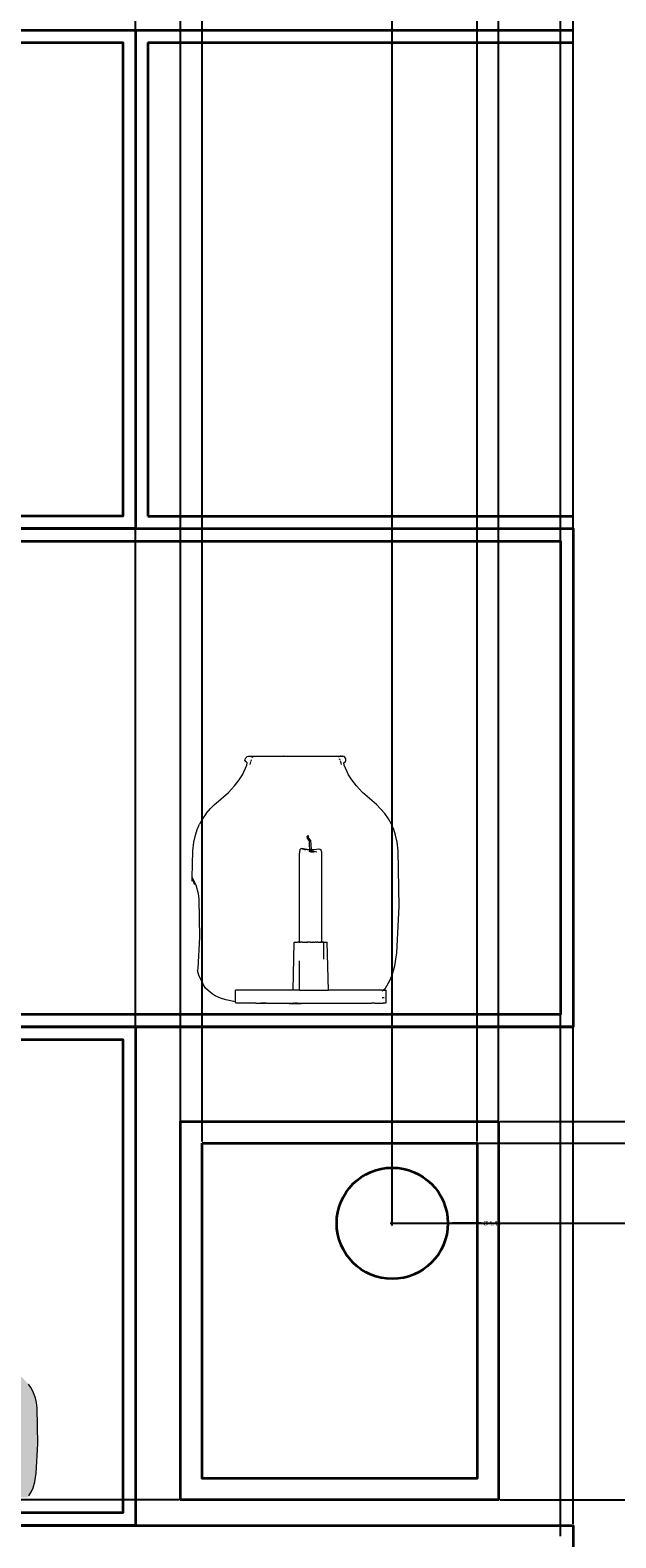
# Model space of a CAD drawing. Units: millimetres. Extents: x 446512 to 447461, y 70395 to 70610.
# Tile 19 of 39: x 446725 to 446748, y 70473 to 70533. Entities that reach past the tile are written whole.
import ezdxf

# ---------------------------------------------------------------- set-up
doc = ezdxf.new("R2010")
doc.units = ezdxf.units.MM
for name, color, linetype, lineweight in [('A-ANNO-DIMS', 2, 'Continuous', 18), ('A-FURN', 7, 'Continuous', 35), ('A-FURN-DECO', 8, 'Continuous', 13), ('A-FURN-PATT', 38, 'Continuous', 13)]:
    doc.layers.add(name, color=color, linetype=linetype, lineweight=lineweight)
doc.styles.get("Standard").update_dxf_attribs({"font": 'arial.ttf'})
doc.dimstyles.get("Standard").update_dxf_attribs({"dimtxt": 0.18, "dimasz": 0.18, "dimexe": 0.18, "dimexo": 0.0625, "dimgap": 0.09, "dimtad": 0, "dimtih": 1, "dimtoh": 1, "dimdec": 4, "dimzin": 0, "dimdsep": 46, "dimtxsty": 'Standard', "dimcen": 0.09, "dimadec": 0, "dimazin": 0, "dimtfac": 1, "dimtdec": 4, "dimtofl": 0, "dimtmove": 0, "dimatfit": 3, "dimfxl": 1, "dimtolj": 1, "dimtzin": 0, "dimarcsym": 0})

# ---------------------------------------------------------------- blocks, each defined once
blk = doc.blocks.new('DECO-VASE-B')
for p, q in [((2.121, 9.752), (2.128, 9.807)), ((2.121, 9.752), (2.136, 9.719)), ((2.128, 9.807), (2.158, 9.87)), ((2.184, 9.693), (2.136, 9.719)), ((2.158, 9.87), (2.204, 9.914)), ((2.208, 9.658), (2.184, 9.693)), ((2.204, 9.914), (2.257, 9.937)), ((2.257, 9.937), (2.375, 9.928)), ((2.257, 9.937), (3.651, 9.937)), ((2.34, 9.701), (2.323, 9.65)), ((2.369, 9.787), (2.35, 9.732)), ((2.375, 9.928), (2.419, 9.892)), ((2.419, 9.892), (2.422, 9.871)), ((3.666, 9.936), (3.651, 9.937)), ((3.666, 9.936), (5.973, 9.937)), ((5.872, 9.93), (5.946, 9.933)), ((5.899, 9.917), (5.879, 9.893)), ((5.891, 9.829), (5.92, 9.807)), ((5.946, 9.933), (5.899, 9.917)), ((5.92, 9.807), (5.927, 9.787)), ((5.944, 9.737), (5.948, 9.727)), ((5.973, 9.937), (5.946, 9.933)), ((5.954, 9.711), (5.974, 9.652)), ((5.977, 9.937), (5.973, 9.937)), ((5.977, 9.937), (6.043, 9.936)), ((6.097, 9.911), (6.043, 9.936)), ((6.151, 9.85), (6.097, 9.911)), ((6.097, 9.677), (6.158, 9.717)), ((6.169, 9.807), (6.151, 9.85)), ((6.158, 9.717), (6.174, 9.743)), ((6.174, 9.743), (6.169, 9.807)), ((1.892, 8.976), (2.026, 9.184)), ((2.026, 9.184), (2.196, 9.575)), ((2.196, 9.575), (2.208, 9.658)), ((2.323, 9.65), (2.313, 9.594)), ((5.974, 9.652), (5.984, 9.593)), ((6.088, 9.658), (6.097, 9.677)), ((6.101, 9.575), (6.088, 9.658)), ((6.27, 9.184), (6.101, 9.575)), ((6.405, 8.976), (6.27, 9.184)), ((0.966, 8.05), (1.454, 8.473)), ((1.454, 8.473), (1.704, 8.737)), ((1.704, 8.737), (1.892, 8.976)), ((6.592, 8.737), (6.405, 8.976)), ((6.842, 8.473), (6.592, 8.737)), ((7.4, 7.989), (6.842, 8.473)), ((0.741, 7.837), (0.896, 7.989)), ((0.896, 7.989), (0.966, 8.05)), ((7.734, 7.63), (7.4, 7.989)), ((0.415, 7.419), (0.296, 7.204)), ((0.562, 7.63), (0.415, 7.419)), ((0.562, 7.63), (0.741, 7.837)), ((7.882, 7.419), (7.734, 7.63)), ((8.001, 7.204), (7.882, 7.419)), ((0.066, 6.478), (0.13, 6.762)), ((0.13, 6.762), (0.202, 6.985)), ((0.202, 6.985), (0.296, 7.204)), ((4.665, 6.727), (4.616, 6.724)), ((4.628, 6.627), (4.616, 6.724)), ((4.676, 6.66), (4.665, 6.727)), ((4.753, 6.557), (4.676, 6.66)), ((8.095, 6.985), (8.001, 7.204)), ((8.167, 6.762), (8.095, 6.985)), ((8.23, 6.478), (8.167, 6.762)), ((0.003, 5.065), (0.022, 6.129)), ((0.022, 6.129), (0.066, 6.478)), ((4.307, 5.974), (4.332, 6.194)), ((4.392, 6.222), (4.332, 6.194)), ((4.611, 6.182), (4.392, 6.222)), ((4.567, 6.159), (4.412, 6.207)), ((4.412, 6.207), (4.611, 6.182)), ((4.611, 6.182), (4.719, 6.182)), ((4.72, 6.153), (4.611, 6.182)), ((4.711, 6.536), (4.628, 6.627)), ((4.721, 6.111), (4.691, 6.12)), ((4.714, 6.371), (4.711, 6.536)), ((4.719, 6.182), (4.714, 6.371)), ((4.72, 6.153), (4.719, 6.182)), ((4.719, 6.182), (4.779, 6.182)), ((4.782, 6.137), (4.72, 6.153)), ((4.72, 6.143), (4.72, 6.149)), ((4.721, 6.111), (4.721, 6.13)), ((4.752, 6.101), (4.721, 6.111)), ((4.722, 6.089), (4.721, 6.111)), ((4.761, 6.087), (4.722, 6.089)), ((4.752, 6.101), (4.784, 6.098)), ((4.753, 6.557), (4.779, 6.182)), ((4.761, 6.087), (4.785, 6.086)), ((4.779, 6.182), (4.782, 6.137)), ((4.779, 6.182), (4.892, 6.182)), ((5.006, 6.08), (4.782, 6.137)), ((4.782, 6.129), (4.783, 6.109)), ((4.784, 6.098), (4.785, 6.086)), ((4.784, 6.098), (4.899, 6.089)), ((4.892, 6.182), (5.091, 6.212)), ((5.091, 6.212), (5.171, 6.181)), ((5.19, 6.109), (5.171, 6.181)), ((5.19, 6.109), (5.194, 2.461)), ((8.274, 6.129), (8.23, 6.478)), ((8.315, 3.894), (8.274, 6.129)), ((4.307, 2.461), (4.307, 5.974)), ((0, 4.992), (0.003, 5.065)), ((0.002, 4.989), (0, 4.992)), ((0, 4.911), (0.002, 4.989)), ((0.057, 4.898), (0.002, 4.989)), ((0.003, 5.065), (0.148, 4.769)), ((0.105, 4.769), (0.057, 4.898)), ((0.148, 4.769), (0.24, 4.424)), ((0.24, 4.424), (0.27, 4.187)), ((0.27, 4.187), (0.298, 2.664)), ((8.221, 2.044), (8.315, 3.894)), ((0.298, 2.664), (0.234, 1.404)), ((4.054, 0.538), (4.098, 2.454)), ((4.098, 2.454), (4.106, 2.461)), ((4.106, 2.461), (4.163, 2.461)), ((4.163, 2.461), (4.167, 2.461)), ((4.167, 2.461), (4.192, 2.461)), ((4.192, 2.461), (4.198, 2.461)), ((4.198, 2.461), (4.201, 2.461)), ((4.201, 2.461), (4.218, 2.461)), ((4.218, 2.461), (4.227, 2.461)), ((4.227, 2.461), (4.232, 2.461)), ((4.232, 2.461), (4.235, 2.461)), ((4.235, 2.461), (4.239, 2.461)), ((4.239, 2.461), (4.246, 2.461)), ((4.25, 2.461), (4.246, 2.461)), ((4.246, 2.461), (4.246, 2.454)), ((4.25, 2.461), (4.253, 2.461)), ((4.253, 2.461), (4.261, 2.461)), ((4.274, 2.461), (4.261, 2.461)), ((4.278, 2.461), (4.274, 2.461)), ((4.278, 2.461), (4.29, 2.461)), ((4.29, 2.461), (4.293, 2.461)), ((4.293, 2.461), (4.295, 2.461)), ((4.295, 2.461), (4.307, 2.461)), ((4.307, 2.454), (4.307, 2.461)), ((4.323, 2.461), (4.307, 2.461)), ((4.323, 2.461), (4.344, 2.461)), ((4.416, 2.461), (4.344, 2.461)), ((4.427, 2.461), (4.416, 2.461)), ((4.427, 2.461), (4.484, 2.461)), ((4.484, 2.461), (4.498, 2.461)), ((4.498, 2.461), (4.589, 2.461)), ((4.605, 2.461), (4.589, 2.461)), ((4.605, 2.461), (4.638, 2.461)), ((4.732, 2.461), (4.638, 2.461)), ((4.732, 2.461), (4.738, 2.461)), ((4.738, 2.461), (4.839, 2.461)), ((4.861, 2.461), (4.839, 2.461)), ((4.861, 2.461), (4.924, 2.461)), ((4.924, 2.461), (4.937, 2.461)), ((4.973, 2.461), (4.937, 2.461)), ((4.978, 2.461), (4.973, 2.461)), ((4.983, 2.461), (4.978, 2.461)), ((4.983, 2.461), (4.987, 2.461)), ((4.987, 2.461), (4.99, 2.461)), ((4.99, 2.461), (5.024, 2.461)), ((5.037, 2.461), (5.024, 2.461)), ((5.064, 2.461), (5.037, 2.461)), ((5.064, 2.461), (5.07, 2.461)), ((5.07, 2.461), (5.144, 2.461)), ((5.154, 2.461), (5.144, 2.461)), ((5.154, 2.461), (5.181, 2.461)), ((5.188, 2.461), (5.181, 2.461)), ((5.194, 2.461), (5.188, 2.461)), ((5.194, 2.461), (5.194, 2.454)), ((5.196, 2.461), (5.194, 2.461)), ((5.202, 2.461), (5.196, 2.461)), ((5.204, 2.461), (5.202, 2.461)), ((5.204, 2.461), (5.219, 2.461)), ((5.224, 2.461), (5.219, 2.461)), ((5.244, 2.461), (5.224, 2.461)), ((5.249, 2.461), (5.244, 2.461)), ((5.249, 2.461), (5.262, 2.461)), ((5.276, 2.461), (5.262, 2.461)), ((5.276, 2.461), (5.266, 1.782)), ((5.28, 2.461), (5.276, 2.461)), ((5.285, 2.461), (5.28, 2.461)), ((5.285, 2.461), (5.312, 2.461)), ((5.312, 2.461), (5.318, 2.461)), ((5.318, 2.461), (5.325, 2.461)), ((5.325, 2.461), (5.348, 2.461)), ((5.348, 2.461), (5.351, 2.461)), ((5.351, 2.461), (5.355, 2.461)), ((5.355, 2.461), (5.365, 2.461)), ((5.365, 2.461), (5.415, 2.461)), ((5.423, 2.454), (5.415, 2.461)), ((5.467, 0.538), (5.423, 2.454)), ((8.128, 1.516), (8.221, 2.044)), ((0.234, 1.404), (0.221, 1.331)), ((0.275, 1.141), (0.221, 1.331)), ((4.307, 0.538), (4.307, 1.712)), ((8.022, 1.141), (8.128, 1.516)), ((0.453, 0.752), (0.275, 1.141)), ((0.54, 0.627), (0.453, 0.752)), ((0.637, 0.522), (0.54, 0.627)), ((7.662, 0.538), (7.756, 0.627)), ((7.756, 0.627), (7.921, 0.896)), ((7.921, 0.896), (8.022, 1.141)), ((0.804, 0.392), (0.637, 0.522)), ((0.929, 0.318), (0.804, 0.392)), ((1.134, 0.226), (0.929, 0.318)), ((1.358, 0.154), (1.134, 0.226)), ((1.679, 0.085), (1.358, 0.154)), ((1.734, 0.078), (1.679, 0.085)), ((1.734, 0.266), (1.734, 0.538)), ((4.054, 0.538), (1.734, 0.538)), ((1.734, 0.078), (1.734, 0.266)), ((1.734, 0.049), (1.734, 0.078)), ((1.757, 0.021), (1.734, 0.049)), ((2.515, 0.021), (1.757, 0.021)), ((2.539, 0.023), (2.515, 0.021)), ((2.551, 0.021), (2.539, 0.023)), ((2.551, 0.021), (2.948, 0.021)), ((2.948, 0.021), (2.761, 0.023)), ((2.969, 0.024), (2.948, 0.021)), ((2.991, 0.021), (2.969, 0.024)), ((2.991, 0.021), (4.067, 0.021)), ((3.896, 0), (4.077, 0.018)), ((4.307, 0.538), (4.054, 0.538)), ((4.077, 0.018), (4.067, 0.021)), ((4.077, 0.018), (4.126, 0.021)), ((4.176, 0.018), (4.126, 0.021)), ((4.196, 0.021), (4.176, 0.018)), ((4.196, 0.021), (4.248, 0.018)), ((4.248, 0.018), (4.27, 0.021)), ((4.392, 0), (4.248, 0.018)), ((4.27, 0.021), (7.006, 0.021)), ((4.307, 0.538), (5.467, 0.538)), ((7.621, 0.538), (5.467, 0.538)), ((7.006, 0.021), (7.192, 0.022)), ((7.325, 0.021), (7.192, 0.022)), ((7.325, 0.021), (7.349, 0.022)), ((7.349, 0.022), (7.351, 0.022)), ((7.349, 0.022), (7.353, 0.022)), ((7.353, 0.022), (7.467, 0.021)), ((7.467, 0.021), (7.488, 0.022)), ((7.488, 0.022), (7.49, 0.022)), ((7.49, 0.022), (7.582, 0.021)), ((7.582, 0.021), (7.645, 0.021)), ((7.621, 0.499), (7.662, 0.538)), ((7.621, 0.538), (7.662, 0.538)), ((7.645, 0.021), (7.67, 0.021)), ((7.675, 0.538), (7.662, 0.538)), ((7.683, 0.021), (7.67, 0.021)), ((7.692, 0.538), (7.675, 0.538)), ((7.765, 0.021), (7.683, 0.021)), ((7.692, 0.538), (7.787, 0.538)), ((7.765, 0.021), (7.788, 0.049)), ((7.788, 0.049), (7.787, 0.538)), ((3.896, 0), (4.392, 0))]:
    blk.add_line(p, q)
blk = doc.blocks.new('*D29')
at = {"layer": 'A-ANNO-DIMS', "color": 0, "lineweight": -2, "transparency": 16777216}
for p, q in [((446730.822, 70489.647), (446730.822, 70578.175)), ((446743.582, 70489.647), (446743.582, 70578.175)), ((446731.002, 70577.995), (446736.817, 70577.995)), ((446743.402, 70577.995), (446737.587, 70577.995))]:
    blk.add_line(p, q, dxfattribs=at)
at = {"layer": 'A-ANNO-DIMS', "color": 0, "transparency": 16777216}
for points in [[(446731.002, 70578.025), (446731.002, 70577.965), (446730.822, 70577.995)], [(446743.402, 70578.025), (446743.402, 70577.965), (446743.582, 70577.995)]]:
    blk.add_solid(points, dxfattribs=at)
at = {"layer": 'Defpoints', "color": 0, "transparency": 16777216}
for p in [(446743.582, 70577.995), (446730.822, 70489.584), (446743.582, 70489.584)]:
    blk.add_point(p, dxfattribs=at)
at = {"layer": 'A-ANNO-DIMS', "color": 0, "transparency": 16777216, "insert": (446737.202, 70577.995), "char_height": 0.18, "attachment_point": 5}
blk.add_mtext('\\A1;12.76', dxfattribs=at)
blk = doc.blocks.new('*D30')
at = {"layer": 'A-ANNO-DIMS', "color": 0, "lineweight": -2, "transparency": 16777216}
for p, q in [((446743.644, 70489.584), (446787.753, 70489.584)), ((446787.573, 70489.404), (446787.573, 70482.176)), ((446787.573, 70474.585), (446787.573, 70481.813)), ((446743.644, 70474.405), (446787.753, 70474.405))]:
    blk.add_line(p, q, dxfattribs=at)
at = {"layer": 'A-ANNO-DIMS', "color": 0, "transparency": 16777216}
for points in [[(446787.543, 70489.404), (446787.603, 70489.404), (446787.573, 70489.584)], [(446787.543, 70474.585), (446787.603, 70474.585), (446787.573, 70474.405)]]:
    blk.add_solid(points, dxfattribs=at)
at = {"layer": 'Defpoints', "color": 0, "transparency": 16777216}
for p in [(446743.582, 70489.584), (446787.573, 70489.584), (446743.582, 70474.405)]:
    blk.add_point(p, dxfattribs=at)
at = {"layer": 'A-ANNO-DIMS', "color": 0, "transparency": 16777216, "insert": (446787.573, 70481.995), "char_height": 0.18, "attachment_point": 5}
blk.add_mtext('\\A1;15.18', dxfattribs=at)
blk = doc.blocks.new('*D31')
at = {"layer": 'A-ANNO-DIMS', "color": 0, "lineweight": -2, "transparency": 16777216}
for p, q in [((446729.008, 70473.444), (446729.008, 70578.175)), ((446730.822, 70474.467), (446730.822, 70578.175)), ((446729.188, 70577.995), (446729.531, 70577.995)), ((446730.642, 70577.995), (446730.3, 70577.995))]:
    blk.add_line(p, q, dxfattribs=at)
at = {"layer": 'A-ANNO-DIMS', "color": 0, "transparency": 16777216}
for points in [[(446729.188, 70578.025), (446729.188, 70577.965), (446729.008, 70577.995)], [(446730.642, 70578.025), (446730.642, 70577.965), (446730.822, 70577.995)]]:
    blk.add_solid(points, dxfattribs=at)
at = {"layer": 'Defpoints', "color": 0, "transparency": 16777216}
for p in [(446730.822, 70577.995), (446730.822, 70474.405), (446729.008, 70473.382)]:
    blk.add_point(p, dxfattribs=at)
at = {"layer": 'A-ANNO-DIMS', "color": 0, "transparency": 16777216, "insert": (446729.915, 70577.995), "char_height": 0.18, "attachment_point": 5}
blk.add_mtext('\\A1;1.814', dxfattribs=at)
blk = doc.blocks.new('*D32')
at = {"layer": 'A-ANNO-DIMS', "color": 0, "lineweight": -2, "transparency": 16777216}
for p, q in [((446730.76, 70474.405), (446678.043, 70474.405)), ((446678.223, 70474.225), (446678.223, 70474.075)), ((446678.223, 70473.562), (446678.223, 70473.711)), ((446728.946, 70473.382), (446678.043, 70473.382))]:
    blk.add_line(p, q, dxfattribs=at)
at = {"layer": 'A-ANNO-DIMS', "color": 0, "transparency": 16777216}
for points in [[(446678.193, 70474.225), (446678.253, 70474.225), (446678.223, 70474.405)], [(446678.193, 70473.562), (446678.253, 70473.562), (446678.223, 70473.382)]]:
    blk.add_solid(points, dxfattribs=at)
at = {"layer": 'Defpoints', "color": 0, "transparency": 16777216}
for p in [(446730.822, 70474.405), (446678.223, 70473.382), (446729.008, 70473.382)]:
    blk.add_point(p, dxfattribs=at)
at = {"layer": 'A-ANNO-DIMS', "color": 0, "transparency": 16777216, "insert": (446678.223, 70473.893), "char_height": 0.18, "attachment_point": 5}
blk.add_mtext('\\A1;1.02', dxfattribs=at)
blk = doc.blocks.new('*D33')
at = {"layer": 'A-ANNO-DIMS', "color": 0, "lineweight": -2, "transparency": 16777216}
for p, q in [((446730.822366, 70489.64696), (446730.822366, 70578.17492)), ((446731.68472, 70488.784606), (446731.68472, 70578.17492)), ((446730.642366, 70577.99492), (446730.462366, 70577.99492)), ((446731.86472, 70577.99492), (446732.04472, 70577.99492))]:
    blk.add_line(p, q, dxfattribs=at)
at = {"layer": 'A-ANNO-DIMS', "color": 0, "transparency": 16777216}
for points in [[(446730.642366, 70578.02492), (446730.642366, 70577.96492), (446730.822366, 70577.99492)], [(446731.86472, 70578.02492), (446731.86472, 70577.96492), (446731.68472, 70577.99492)]]:
    blk.add_solid(points, dxfattribs=at)
at = {"layer": 'Defpoints', "color": 0, "transparency": 16777216}
for p in [(446731.68472, 70577.99492), (446730.822366, 70489.58446), (446731.68472, 70488.722106)]:
    blk.add_point(p, dxfattribs=at)
at = {"layer": 'A-ANNO-DIMS', "color": 0, "transparency": 16777216, "insert": (446731.253543, 70577.99492), "char_height": 0.18, "attachment_point": 5}
blk.add_mtext('\\A1;0.86', dxfattribs=at)
blk = doc.blocks.new('*D34')
at = {"layer": 'A-ANNO-DIMS', "color": 0, "lineweight": -2, "transparency": 16777216}
for p, q in [((446739.318, 70485.567), (446739.318, 70578.175)), ((446742.719, 70488.785), (446742.719, 70578.175)), ((446739.498, 70577.995), (446740.642, 70577.995)), ((446742.539, 70577.995), (446741.395, 70577.995))]:
    blk.add_line(p, q, dxfattribs=at)
at = {"layer": 'A-ANNO-DIMS', "color": 0, "transparency": 16777216}
for points in [[(446739.498, 70578.025), (446739.498, 70577.965), (446739.318, 70577.995)], [(446742.539, 70578.025), (446742.539, 70577.965), (446742.719, 70577.995)]]:
    blk.add_solid(points, dxfattribs=at)
at = {"layer": 'Defpoints', "color": 0, "transparency": 16777216}
for p in [(446739.318, 70577.995), (446742.719, 70488.722), (446739.318, 70485.504)]:
    blk.add_point(p, dxfattribs=at)
at = {"layer": 'A-ANNO-DIMS', "color": 0, "transparency": 16777216, "insert": (446741.019, 70577.995), "char_height": 0.18, "attachment_point": 5}
blk.add_mtext('\\A1;3.401', dxfattribs=at)
blk = doc.blocks.new('*D35')
at = {"layer": 'A-ANNO-DIMS', "color": 0, "lineweight": -2, "transparency": 16777216}
for p, q in [((446742.782, 70488.722), (446787.753, 70488.722)), ((446787.573, 70488.542), (446787.573, 70487.295)), ((446787.573, 70485.684), (446787.573, 70486.931)), ((446739.381, 70485.504), (446787.753, 70485.504))]:
    blk.add_line(p, q, dxfattribs=at)
at = {"layer": 'A-ANNO-DIMS', "color": 0, "transparency": 16777216}
for points in [[(446787.543, 70488.542), (446787.603, 70488.542), (446787.573, 70488.722)], [(446787.543, 70485.684), (446787.603, 70485.684), (446787.573, 70485.504)]]:
    blk.add_solid(points, dxfattribs=at)
at = {"layer": 'Defpoints', "color": 0, "transparency": 16777216}
for p in [(446742.719, 70488.722), (446739.318, 70485.504), (446787.573, 70485.504)]:
    blk.add_point(p, dxfattribs=at)
at = {"layer": 'A-ANNO-DIMS', "color": 0, "transparency": 16777216, "insert": (446787.573, 70487.113), "char_height": 0.18, "attachment_point": 5}
blk.add_mtext('\\A1;3.22', dxfattribs=at)
blk = doc.blocks.new('*D36')
at = {"layer": 'A-ANNO-DIMS', "color": 0, "lineweight": -2, "transparency": 16777216}
for p, q in [((446746.073, 70472.944), (446746.073, 70578.175)), ((446746.573, 70473.444), (446746.573, 70578.175)), ((446745.893, 70577.995), (446745.713, 70577.995)), ((446746.753, 70577.995), (446746.933, 70577.995))]:
    blk.add_line(p, q, dxfattribs=at)
at = {"layer": 'A-ANNO-DIMS', "color": 0, "transparency": 16777216}
for points in [[(446745.893, 70578.025), (446745.893, 70577.965), (446746.073, 70577.995)], [(446746.753, 70578.025), (446746.753, 70577.965), (446746.573, 70577.995)]]:
    blk.add_solid(points, dxfattribs=at)
at = {"layer": 'Defpoints', "color": 0, "transparency": 16777216}
for p in [(446746.573, 70577.995), (446746.073, 70472.882), (446746.573, 70473.382)]:
    blk.add_point(p, dxfattribs=at)
at = {"layer": 'A-ANNO-DIMS', "color": 0, "transparency": 16777216, "insert": (446747.187, 70577.995), "char_height": 0.18, "attachment_point": 5}
blk.add_mtext('\\A1;0.5', dxfattribs=at)
blk = doc.blocks.new('*D78')
at = {"layer": 'A-ANNO-DIMS', "color": 0, "lineweight": -2, "transparency": 16777216}
for p, q in [((446739.318, 70485.414), (446739.318, 70485.594)), ((446739.228, 70485.504), (446739.408, 70485.504)), ((446742.886, 70485.504), (446741.728, 70485.504))]:
    blk.add_line(p, q, dxfattribs=at)
at = {"layer": 'A-ANNO-DIMS', "color": 0, "transparency": 16777216}
blk.add_solid([(446741.728, 70485.534), (446741.728, 70485.474), (446741.548, 70485.504)], dxfattribs=at)
at = {"layer": 'Defpoints', "color": 0, "transparency": 16777216}
for p in [(446737.088, 70485.505), (446741.548, 70485.504)]:
    blk.add_point(p, dxfattribs=at)
at = {"layer": 'A-ANNO-DIMS', "color": 0, "transparency": 16777216, "insert": (446743.308, 70485.504), "char_height": 0.18, "attachment_point": 5}
blk.add_mtext('\\A1;∅4.46', dxfattribs=at)

msp = doc.modelspace()

# ---------------------------------------------------------------- hatches: boundary and pattern name
at = {"layer": 'A-FURN-PATT'}
h = msp.add_hatch(color=256, dxfattribs=at)
h.dxf.hatch_style = 1
h.paths.add_polyline_path([(446703.5722, 70477.5476), (446703.5295, 70477.5904), (446703.508, 70477.5904), (446703.383, 70477.6041), (446703.3062, 70477.6039), (446702.8621, 70477.6193), (446702.7177, 70477.6193), (446702.6174, 70477.6163), (446702.576, 70477.615), (446702.5757, 70477.6192), (446702.3373, 70477.6192), (446701.7238, 70477.5898), (446701.6039, 70477.5792), (446701.5612, 70477.5357), (446701.547, 70474.1653), (446703.5225, 70474.1653), (446703.5865, 70474.1653), (446703.5861, 70474.2632), (446703.5852, 70474.4594)])
h.paths.add_polyline_path([(446715.9764, 70475.5286), (446716.1565, 70476.0766), (446716.2492, 70476.4728), (446716.2873, 70476.8422), (446716.2666, 70477.0104), (446716.236, 70477.1061), (446716.1173, 70477.332), (446715.9979, 70477.4937), (446715.8249, 70477.6853), (446715.558, 70477.9316), (446715.2321, 70478.1882), (446714.7182, 70478.5467), (446714.5954, 70478.6535), (446714.3996, 70478.8999), (446714.3461, 70479.0185), (446714.3253, 70479.1028), (446714.3286, 70480.1095), (446714.368, 70480.1364), (446714.3744, 70480.152), (446714.3709, 70480.1808), (446714.3551, 70480.2131), (446714.3271, 70480.2359), (446714.3039, 70480.2478), (446714.2782, 70480.2478), (446714.259, 70480.2458), (446714.2432, 70480.2391), (446714.2375, 70480.2284), (446714.2369, 70480.2218), (446714.2301, 70480.2478), (446713.8255, 70480.2478), (446713.8277, 70480.2375), (446713.8104, 70480.2458), (446713.7912, 70480.2478), (446713.7655, 70480.2478), (446713.738, 70480.2359), (446713.7079, 70480.2028), (446713.6947, 70480.1567), (446713.6986, 70480.1448), (446713.717, 70480.1274), (446713.7341, 70480.1112), (446713.7407, 70480.1049), (446713.7473, 70479.1348), (446713.7233, 70479.0185), (446713.6698, 70478.8999), (446713.5684, 70478.7546), (446713.4739, 70478.6535), (446713.3511, 70478.5467), (446712.8373, 70478.1882), (446712.5114, 70477.9316), (446712.4629, 70477.8868), (446712.2445, 70477.6853), (446712.0714, 70477.4937), (446711.9521, 70477.332), (446711.866, 70477.1682), (446711.8333, 70477.1061), (446711.7899, 70476.9473), (446711.7821, 70476.8422), (446711.8202, 70476.4728), (446711.8563, 70476.3184), (446711.9128, 70476.0766), (446712.093, 70475.5286), (446712.2916, 70475.0627), (446712.4529, 70474.7607), (446712.5622, 70474.5947), (446712.6434, 70474.4935), (446712.7522, 70474.3925), (446712.8451, 70474.3334), (446713.0597, 70474.2483), (446713.2189, 70474.2124), (446713.4296, 70474.1861), (446713.8128, 70474.1834), (446713.5915, 70474.1683), (446714.5392, 70474.1683), (446714.4414, 70474.1779), (446714.1836, 70474.1834), (446714.6098, 70474.1861), (446714.8353, 70474.2124), (446714.9266, 70474.2312), (446715.0097, 70474.2483), (446715.2243, 70474.3334), (446715.3172, 70474.3925), (446715.3727, 70474.4388), (446715.5072, 70474.5947), (446715.6164, 70474.7607), (446715.7778, 70475.0627)])
h.paths.add_polyline_path([(446719.9646, 70475.8685), (446719.9469, 70476.8426), (446719.9277, 70476.9944), (446719.8688, 70477.2155), (446719.7757, 70477.4048), (446719.7115, 70477.4967), (446719.566, 70477.6531), (446719.2165, 70477.9493), (446719.1289, 70478.0481), (446719.1777, 70478.067), (446719.1866, 70478.0815), (446719.1867, 70478.209), (446719.1598, 70478.218), (446719.1369, 70478.2173), (446719.1374, 70478.2174), (446719.0341, 70478.2174), (446718.8666, 70478.218), (446718.6447, 70478.218), (446718.418, 70478.2174), (446718.1448, 70478.2174), (446717.8911, 70478.218), (446717.8873, 70478.218), (446717.6401, 70478.2174), (446717.4215, 70478.2174), (446717.2754, 70478.218), (446717.1987, 70478.218), (446717.2097, 70478.2113), (446717.1243, 70478.2174), (446717.1135, 70478.2124), (446717.1091, 70478.2029), (446717.1111, 70478.0815), (446717.1185, 70478.0683), (446717.1615, 70478.0517), (446717.1433, 70478.0167), (446717.0812, 70477.9493), (446716.7317, 70477.6531), (446716.5862, 70477.4967), (446716.47, 70477.311), (446716.3975, 70477.1183), (446716.37, 70476.9944), (446716.3508, 70476.8426), (446716.3331, 70475.8685), (446716.374, 70475.0624), (446716.4146, 70474.8322), (446716.4608, 70474.6687), (446716.5046, 70474.5619), (446716.5765, 70474.4449), (446716.6659, 70474.36), (446716.7457, 70474.3103), (446716.8351, 70474.2702), (446717.0729, 70474.2085), (446717.2886, 70474.1864), (446717.3803, 70474.1864), (446717.4428, 70474.1846), (446717.4556, 70474.1862), (446718.0146, 70474.1842), (446718.1072, 70474.1795), (446718.1371, 70474.1802), (446718.1473, 70474.1804), (446718.1566, 70474.1797), (446718.1569, 70474.1797), (446718.1592, 70474.1795), (446718.303, 70474.1842), (446719.0393, 70474.1865), (446719.2248, 70474.2085), (446719.365, 70474.2387), (446719.4626, 70474.2702), (446719.552, 70474.3103), (446719.6318, 70474.36), (446719.7212, 70474.4449), (446719.7931, 70474.5619), (446719.8369, 70474.6687), (446719.8831, 70474.8322), (446719.9155, 70475.0156), (446719.9237, 70475.0624)])
h.paths.add_polyline_path([(446718.18, 70474.3158), (446717.2692, 70474.3158), (446717.2092, 70474.3107), (446717.3763, 70474.3107)], flags=16)
h.paths.add_polyline_path([(446717.572, 70474.3384), (446717.5676, 70474.3381), (446717.5691, 70474.3381)], flags=16)
h.paths.add_polyline_path([(446722.3965, 70475.7383), (446722.4453, 70475.7383), (446722.4564, 70475.7383), (446722.4729, 70475.7383), (446722.4785, 70475.7384), (446722.4797, 70475.7383), (446722.4831, 70475.7383), (446722.4841, 70475.7384), (446722.5211, 70475.7384), (446722.4906, 70475.7381), (446722.4906, 70475.7384), (446722.4864, 70475.7383), (446722.4853, 70475.7383), (446722.4831, 70475.7383), (446722.4819, 70475.7383), (446722.4797, 70475.7383), (446722.4618, 70475.7383), (446722.4401, 70475.7383), (446722.4015, 70475.7383), (446722.3964, 70475.7341), (446722.3682, 70474.5084), (446722.5299, 70474.5084), (446723.2721, 70474.5084), (446723.2439, 70475.7341), (446723.2391, 70475.7383), (446723.2067, 70475.7383), (446723.1904, 70475.7383), (446723.1824, 70475.7383), (446723.1499, 70475.7382), (446723.1499, 70475.7384), (446723.1407, 70475.7384), (446723.1819, 70475.7384), (446723.1732, 70475.7384), (446723.1824, 70475.7383), (446723.1957, 70475.7383), (446723.1982, 70475.7383), (446723.2002, 70475.7383), (446723.2067, 70475.7383), (446723.2439, 70475.7383), (446723.2721, 70474.5084), (446724.6768, 70474.5084), (446724.7369, 70474.5652), (446724.8426, 70474.7369), (446724.9068, 70474.8938), (446724.9747, 70475.1338), (446725.0344, 70475.4718), (446725.0943, 70476.6554), (446725.0683, 70478.0856), (446725.0402, 70478.3085), (446724.9998, 70478.4903), (446724.9537, 70478.6331), (446724.8934, 70478.7733), (446724.817, 70478.911), (446724.7228, 70479.046), (446724.5091, 70479.2756), (446724.1522, 70479.5853), (446723.9922, 70479.7544), (446723.8721, 70479.9071), (446723.7862, 70480.0401), (446723.6778, 70480.2901), (446723.6684, 70480.351), (446723.714, 70480.381), (446723.7245, 70480.398), (446723.7213, 70480.4391), (446723.7096, 70480.4663), (446723.6751, 70480.5056), (446723.6405, 70480.5215), (446723.5985, 70480.5218), (446723.5958, 70480.5218), (446722.1196, 70480.5215), (446721.2867, 70480.5218), (446721.2939, 70480.516), (446721.2184, 70480.5218), (446721.1844, 70480.5072), (446721.155, 70480.479), (446721.1354, 70480.4391), (446721.1312, 70480.4035), (446721.1408, 70480.3826), (446721.1891, 70480.3558), (446721.179, 70480.2901), (446721.0706, 70480.0401), (446720.9847, 70479.9071), (446720.8645, 70479.7544), (446720.7046, 70479.5853), (446720.3925, 70479.3145), (446720.3476, 70479.2756), (446720.248, 70479.1783), (446720.134, 70479.046), (446720.0397, 70478.911), (446719.9634, 70478.7733), (446719.9031, 70478.6331), (446719.857, 70478.4903), (446719.8165, 70478.3085), (446719.7884, 70478.0856), (446719.7757, 70477.4048), (446719.8688, 70477.2155), (446719.9277, 70476.9944), (446719.9469, 70476.8426), (446719.9646, 70475.8685), (446719.9237, 70475.0624), (446719.9155, 70475.0156), (446719.9499, 70474.8938), (446720.064, 70474.6452), (446720.1198, 70474.5652), (446720.1819, 70474.4977), (446720.2884, 70474.4145), (446720.3682, 70474.3675), (446720.4995, 70474.3087), (446720.6428, 70474.2625), (446720.8486, 70474.2181), (446720.8834, 70474.214), (446720.8836, 70474.3337), (446720.8838, 70474.5084), (446722.3682, 70474.5084)])
h.paths.add_polyline_path([(446722.5299, 70477.9863), (446722.5458, 70478.1272), (446722.5844, 70478.1453), (446722.7245, 70478.1193), (446722.7937, 70478.1192), (446722.7905, 70478.2404), (446722.7882, 70478.3461), (446722.7354, 70478.4044), (446722.7276, 70478.4661), (446722.759, 70478.4678), (446722.7662, 70478.4254), (446722.8155, 70478.3594), (446722.8317, 70478.1191), (446722.9042, 70478.119), (446723.0314, 70478.1383), (446723.0829, 70478.1185), (446723.0949, 70478.0727), (446723.0974, 70475.7384), (446723.1135, 70475.7383), (446723.104, 70475.7384), (446723.1025, 70475.7384), (446723.0987, 70475.7384), (446723.0974, 70475.7383), (446723.0719, 70475.7383), (446723.018, 70475.7384), (446723.0095, 70475.7382), (446722.9885, 70475.7384), (446722.9576, 70475.7383), (446722.9328, 70475.7384), (446722.9244, 70475.7383), (446722.8841, 70475.7383), (446722.8055, 70475.7384), (446722.802, 70475.7383), (446722.7415, 70475.7384), (446722.7206, 70475.7383), (446722.7104, 70475.7384), (446722.6518, 70475.7384), (446722.6431, 70475.7383), (446722.6067, 70475.7383), (446722.5537, 70475.7384), (446722.5299, 70475.7383)], flags=16)
h.paths.add_polyline_path([(446722.7937, 70478.1192), (446722.8317, 70478.1191), (446722.8336, 70478.0906), (446722.8358, 70478.0578), (446722.7952, 70478.0599), (446722.7946, 70478.0859)], flags=0)
h.paths.add_polyline_path([(446723.5789, 70480.5193), (446723.5569, 70480.5185), (446723.5487, 70480.509)], flags=16)

# ---------------------------------------------------------------- linework, layer by layer
at = {"layer": 'A-FURN'}
for p, q in [((446686.5728, 70533.3815), (446746.5728, 70533.3815)), ((446686.5728, 70533.3815), (446729.0084, 70533.3815)), ((446729.0084, 70533.3815), (446729.0084, 70513.3815)), ((446729.0084, 70533.3815), (446729.0084, 70513.3815)), ((446729.5084, 70533.3815), (446746.5728, 70533.3815)), ((446729.5084, 70532.8815), (446729.5084, 70513.8815)), ((446729.5084, 70532.8815), (446746.5728, 70532.8815)), ((446686.5728, 70513.3815), (446746.5728, 70513.3815)), ((446729.0084, 70513.3815), (446686.5728, 70513.3815)), ((446729.5084, 70513.8815), (446746.5728, 70513.8815)), ((446729.5084, 70513.3815), (446746.5728, 70513.3815)), ((446746.5728, 70513.3815), (446746.5728, 70493.3815)), ((446686.5728, 70493.3815), (446746.5728, 70493.3815)), ((446729.0084, 70493.3815), (446729.0084, 70473.3815)), ((446686.5728, 70473.3815), (446746.5728, 70473.3815)), ((446746.5728, 70473.3815), (446746.5728, 70453.3815))]:
    msp.add_line(p, q, dxfattribs=at)
for points in [[(446687.0728, 70532.8815), (446728.5084, 70532.8815), (446728.5084, 70513.8815), (446687.0728, 70513.8815)], [(446699.4288, 70513.3815), (446746.5728, 70513.3815), (446746.5728, 70493.3815), (446699.4288, 70493.3815)], [(446699.9288, 70512.8815), (446746.0728, 70512.8815), (446746.0728, 70493.8815), (446699.9288, 70493.8815)], [(446686.5728, 70493.3815), (446729.0084, 70493.3815), (446729.0084, 70473.3815), (446686.5728, 70473.3815)], [(446687.0728, 70492.8815), (446728.5084, 70492.8815), (446728.5084, 70473.8815), (446687.0728, 70473.8815)], [(446730.8224, 70489.5845), (446743.5815, 70489.5845), (446743.5815, 70474.4047), (446730.8224, 70474.4047)], [(446731.6847, 70488.7221), (446742.7192, 70488.7221), (446742.7192, 70475.2671), (446731.6847, 70475.2671)], [(446699.4288, 70473.3815), (446746.5728, 70473.3815), (446746.5728, 70453.3815), (446699.4288, 70453.3815)]]:
    msp.add_lwpolyline(points, close=True, dxfattribs=at)
msp.add_circle((446739.3181, 70485.5045), 2.2299, dxfattribs=at)
at = {"layer": 'A-FURN-DECO'}
for p, q in [((446738.9654, 70494.55), (446738.9087, 70494.5497)), ((446738.9925, 70494.55), (446738.9654, 70494.55)), ((446724.817, 70478.911), (446724.7228, 70479.046)), ((446724.8934, 70478.7733), (446724.817, 70478.911)), ((446724.9537, 70478.6331), (446724.8934, 70478.7733)), ((446724.9998, 70478.4903), (446724.9537, 70478.6331)), ((446725.0402, 70478.3085), (446724.9998, 70478.4903)), ((446725.0683, 70478.0856), (446725.0402, 70478.3085)), ((446725.0943, 70476.6554), (446725.0683, 70478.0856)), ((446725.0344, 70475.4718), (446725.0943, 70476.6554)), ((446724.9747, 70475.1338), (446725.0344, 70475.4718)), ((446724.7369, 70474.5652), (446724.8426, 70474.7369)), ((446724.8426, 70474.7369), (446724.9068, 70474.8938)), ((446724.9068, 70474.8938), (446724.9747, 70475.1338))]:
    msp.add_line(p, q, dxfattribs=at)

# ---------------------------------------------------------------- block references
msp.add_blockref('DECO-VASE-B', (446731.287, 70494.318), dxfattribs=at)

# ---------------------------------------------------------------- dimensions: what is measured, and where the dimension line sits
at = {"layer": 'A-ANNO-DIMS'}
for base, p1, p2, override, picture, middle in [((446730.8224, 70577.9949), (446729.0084, 70473.3815), (446730.8224, 70474.4047), {"dimdec": 3, "dimlfac": 1, "dimrnd": 0, "dimzin": 0, "dimdsep": 46, "dimlunit": 2}, '*D31', (446729.9154, 70577.9949)), ((446731.6847, 70577.9949), (446730.8224, 70489.5845), (446731.6847, 70488.7221), {"dimdec": 2, "dimlfac": 1, "dimrnd": 0, "dimzin": 0, "dimdsep": 46, "dimlunit": 2}, '*D33', (446731.2535, 70577.9949)), ((446743.5815, 70577.9949), (446730.8224, 70489.5845), (446743.5815, 70489.5845), {"dimdec": 2, "dimlfac": 1, "dimrnd": 0, "dimzin": 0, "dimdsep": 46, "dimlunit": 2}, '*D29', (446737.2019, 70577.9949)), ((446739.3181, 70577.9949), (446742.7192, 70488.7221), (446739.3181, 70485.5045), {"dimdec": 3, "dimlfac": 1, "dimrnd": 0, "dimzin": 0, "dimdsep": 46, "dimlunit": 2}, '*D34', (446741.0186, 70577.9949)), ((446746.5728, 70577.9949), (446746.0728, 70472.8816), (446746.5728, 70473.3815), {"dimdec": 1, "dimlfac": 1, "dimrnd": 0, "dimzin": 0, "dimdsep": 46, "dimlunit": 2}, '*D36', (446747.1874, 70577.9949))]:
    dim = msp.add_linear_dim(base=base, p1=p1, p2=p2, dimstyle='Standard', override=override, dxfattribs=at)
    dim.commit()
    dim.dimension.update_dxf_attribs({"geometry": picture, "text_midpoint": middle})
for base, p1, p2, picture, middle in [((446787.5735, 70489.5845), (446743.5815, 70474.4047), (446743.5815, 70489.5845), '*D30', (446787.5735, 70481.9946)), ((446787.5735, 70485.5045), (446742.7192, 70488.7221), (446739.3181, 70485.5045), '*D35', (446787.5735, 70487.1133)), ((446678.2228, 70473.3815), (446730.8224, 70474.4047), (446729.0084, 70473.3815), '*D32', (446678.2228, 70473.8931))]:
    dim = msp.add_linear_dim(base=base, p1=p1, p2=p2, angle=90, dimstyle='Standard', override={"dimdec": 2, "dimlfac": 1, "dimrnd": 0, "dimzin": 0, "dimdsep": 46, "dimlunit": 2}, dxfattribs=at)
    dim.commit()
    dim.dimension.update_dxf_attribs({"geometry": picture, "text_midpoint": middle})
dim = msp.add_diameter_dim_2p(p1=(446737.0882, 70485.5049), p2=(446741.548, 70485.504), dimstyle='Standard', override={"dimdec": 2, "dimlfac": 1, "dimrnd": 0, "dimzin": 0, "dimdsep": 46, "dimlunit": 2}, dxfattribs=at)
dim.commit()
dim.dimension.update_dxf_attribs({"geometry": '*D78', "text_midpoint": (446742.886, 70485.5037), "dimtype": 163})

doc.saveas('drawing.dxf')
